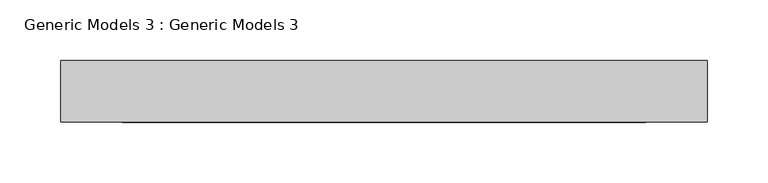
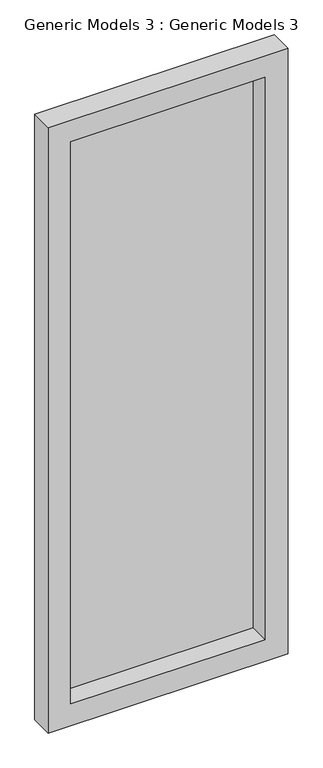
"""IFC4 building model written with IfcOpenShell, lengths in millimetres: proxy geometry, Generic Models 3 : Generic Models 3."""

from ifc_helpers import new_model, si_unit, frame, origin, place, context, project, spatial, polyline, outline, extrude, source, transform, mapped, element, save


def generic_models_3_generic_models_3_c6119d6a(model_context):
    return source(origin(), model_context, "Body", "SweptSolid", [
        extrude(outline(polyline([(-9202.4500083, 1026.6428795), (-9634.2500083, 1026.6428795), (-9634.2500083, 1031.7030358), (-9202.4500083, 1031.7030358), (-9202.4500083, 1026.6428795)])), frame((0.0, 0.0, 4426.8407527), z_axis=(0.0, 0.0, 1.0), x_axis=(1.0, 0.0, 0.0)), (0.0, 0.0, 1.0), 1320.8),
        extrude(outline(polyline([(5798.4407527, -9151.6500083), (5798.4407527, -9685.0500083), (4376.0407527, -9685.0500083), (4376.0407527, -9151.6500083), (5798.4407527, -9151.6500083)]), holes=[polyline([(4426.8407527, -9634.2500083), (5747.6407527, -9634.2500083), (5747.6407527, -9202.4500083), (4426.8407527, -9202.4500083), (4426.8407527, -9634.2500083)])]), frame((0.0, 980.9030358, 0.0), z_axis=(0.0, 1.0, 0.0), x_axis=(0.0, 0.0, 1.0)), (0.0, 0.0, 1.0), 50.8),
    ])


if __name__ == "__main__":
    model = new_model("IFC4")
    model_context = context("Model", 3, world=origin())
    ifc_project = project(units=[si_unit("LENGTHUNIT", "METRE", prefix="MILLI")], contexts=[model_context])
    site = spatial("IfcSite", under=ifc_project)
    building = spatial("IfcBuilding", under=site)
    placement = place(None, origin())
    generic_models_3_generic_models_3_shape = generic_models_3_generic_models_3_c6119d6a(model_context)
    element("IfcBuildingElementProxy", 1, Name="Generic Models 3 : Generic Models 3", ObjectType="Generic Models 3 : Generic Models 3", at=placement, inside=building, context=model_context, shape_type="MappedRepresentation", body=[
        mapped(generic_models_3_generic_models_3_shape, transform((0.0, 0.0, 0.0), x_axis=(1.0, 0.0, 0.0), y_axis=(0.0, 1.0, 0.0), z_axis=(0.0, 0.0, 1.0))),
    ])
    save(model, "model.ifc")

# Revit data of these elements
# Element 1 (IfcBuildingElementProxy, "Generic Models 3 : Generic Models 3")
#   Materials on its faces: "Damp-proofing"
# Materials
#   "Damp-proofing": class "Generic", colour RGB 127 127 127, transparency 0, Description = "Damp-proofing", Cost = 0
